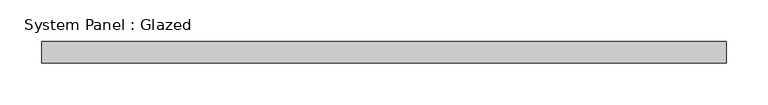
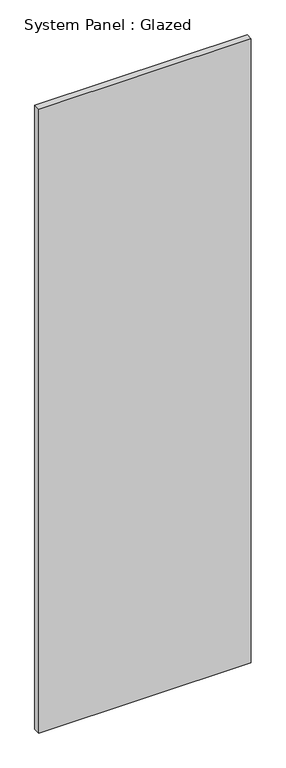
"""IFC4 building model written with IfcOpenShell, lengths in millimetres: plate geometry, System Panel : Glazed."""

from ifc_helpers import new_model, si_unit, origin, origin_with_axes, place, context, project, spatial, polyline, outline, extrude, source, transform, mapped, element, save


def system_panel_glazed_f88502f0(model_context):
    return source(origin(), model_context, "Body", "SweptSolid", [
        extrude(outline(polyline([(409.575, 19.05), (-409.575, 19.05), (-409.575, 44.45), (409.575, 44.45), (409.575, 19.05)])), origin_with_axes(), (0.0, 0.0, 1.0), 2540.0),
    ])


if __name__ == "__main__":
    model = new_model("IFC4")
    model_context = context("Model", 3, world=origin())
    ifc_project = project(units=[si_unit("LENGTHUNIT", "METRE", prefix="MILLI")], contexts=[model_context])
    site = spatial("IfcSite", under=ifc_project)
    building = spatial("IfcBuilding", under=site)
    placement = place(None, origin())
    system_panel_glazed_shape = system_panel_glazed_f88502f0(model_context)
    element("IfcPlate", 1, ObjectType="System Panel : Glazed", at=placement, inside=building, context=model_context, shape_type="MappedRepresentation", body=[
        mapped(system_panel_glazed_shape, transform((0.0, 0.0, 0.0), x_axis=(1.0, 0.0, 0.0), y_axis=(0.0, 1.0, 0.0), z_axis=(0.0, 0.0, 1.0))),
    ])
    save(model, "model.ifc")

# Revit data of these elements
# Type "System Panel : Glazed"
#   Construction Type Id = "GSP4R"
#   Analytic Construction = "1/8 in Pilkington single glazing"
#   Visual Light Transmittance = 0.9
#   Solar Heat Gain Coefficient = 0.86
#   Heat Transfer Coefficient (U) = 1.18115 BTU/(h·ft²·°F)
#   Define Thermal Properties by = 1
# Element 1 (IfcPlate, "System Panel : Glazed")
#   Materials on its faces: "Glass"
# Materials
#   "Glass": class "Glass", colour RGB 0 128 192, transparency 0.75, Description = "Soda Lime Glass", Cost = 0
